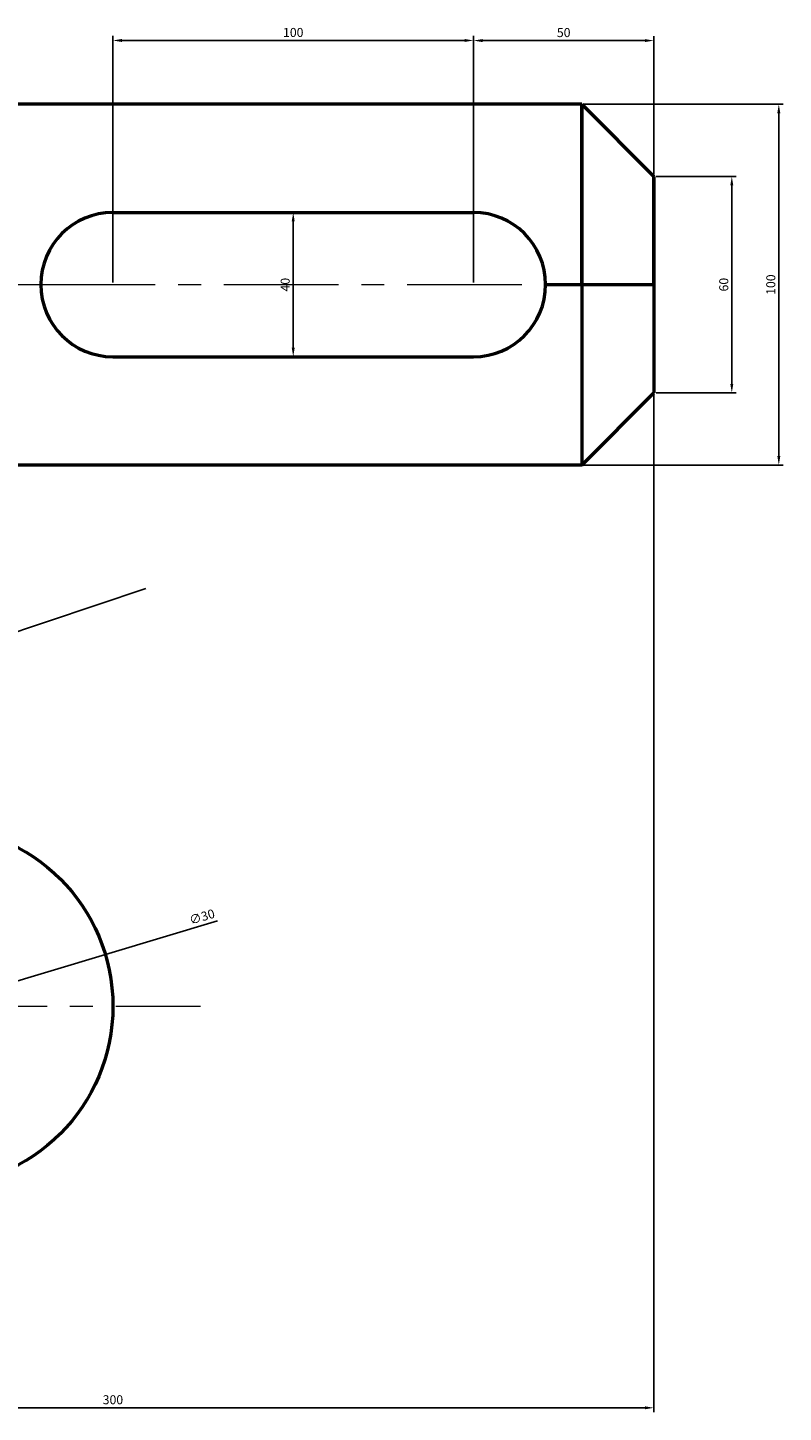
# Model space of a CAD drawing. Units: millimetres. Extents: x 107046 to 107591, y 80056 to 80641.
# Tile 2 of 3: x 107381 to 107591, y 80056 to 80440. Entities that reach past the tile are written whole.
import ezdxf

# ---------------------------------------------------------------- set-up
doc = ezdxf.new("R2010")
doc.units = ezdxf.units.MM
doc.linetypes.add('CENTER', pattern=[50.8, 31.75, -6.35, 6.35, -6.35])
for name, color, linetype, lineweight in [('M-CNTR', 1, 'CENTER', 18), ('M-DIMS', 2, 'Continuous', 25), ('M-OUTL', 7, 'Continuous', 50)]:
    doc.layers.add(name, color=color, linetype=linetype, lineweight=lineweight)
doc.styles.get("Standard").update_dxf_attribs({"font": 'arial.ttf'})
doc.dimstyles.new('ISO-25', dxfattribs={"dimtxt": 2.5, "dimasz": 2.5, "dimexe": 1.25, "dimexo": 0.625, "dimtad": 1, "dimtxsty": 'Standard', "dimcen": 2.5, "dimadec": 0, "dimazin": 0, "dimtfac": 1, "dimtmove": 0, "dimatfit": 3, "dimfxl": 1, "dimarcsym": 0})

# ---------------------------------------------------------------- blocks, each defined once
blk = doc.blocks.new('*D3')
at = {"layer": 'Defpoints', "color": 0, "transparency": 16777216}
for p in [(107255.14, 80368.78), (107555.14, 80368.78), (107555.14, 80057.52)]:
    blk.add_point(p, dxfattribs=at)
at = {"layer": 'M-DIMS', "color": 0, "lineweight": -2, "transparency": 16777216}
for p, q in [((107255.14, 80368.16), (107255.14, 80056.27)), ((107555.14, 80368.16), (107555.14, 80056.27)), ((107257.64, 80057.52), (107552.64, 80057.52))]:
    blk.add_line(p, q, dxfattribs=at)
at = {"layer": 'M-DIMS', "color": 0, "transparency": 16777216}
for points in [[(107257.64, 80057.94), (107257.64, 80057.11), (107255.14, 80057.52)], [(107552.64, 80057.94), (107552.64, 80057.11), (107555.14, 80057.52)]]:
    blk.add_solid(points, dxfattribs=at)
at = {"layer": 'M-DIMS', "color": 0, "transparency": 16777216, "insert": (107405.14, 80059.43), "char_height": 2.5, "attachment_point": 5}
blk.add_mtext('300', dxfattribs=at)
blk = doc.blocks.new('*D4')
at = {"layer": 'Defpoints', "color": 0, "transparency": 16777216}
for p in [(107505.14, 80436.44), (107405.14, 80368.78), (107505.14, 80368.78)]:
    blk.add_point(p, dxfattribs=at)
at = {"layer": 'M-DIMS', "color": 0, "lineweight": -2, "transparency": 16777216}
for p, q in [((107405.14, 80369.41), (107405.14, 80437.69)), ((107505.14, 80369.41), (107505.14, 80437.69)), ((107407.64, 80436.44), (107502.64, 80436.44))]:
    blk.add_line(p, q, dxfattribs=at)
at = {"layer": 'M-DIMS', "color": 0, "transparency": 16777216}
for points in [[(107407.64, 80436.86), (107407.64, 80436.03), (107405.14, 80436.44)], [(107502.64, 80436.86), (107502.64, 80436.03), (107505.14, 80436.44)]]:
    blk.add_solid(points, dxfattribs=at)
at = {"layer": 'M-DIMS', "color": 0, "transparency": 16777216, "insert": (107455.14, 80438.34), "char_height": 2.5, "attachment_point": 5}
blk.add_mtext('100', dxfattribs=at)
blk = doc.blocks.new('*D5')
at = {"layer": 'Defpoints', "color": 0, "transparency": 16777216}
for p in [(107455.14, 80388.78), (107455.14, 80348.78), (107455.14, 80348.78)]:
    blk.add_point(p, dxfattribs=at)
at = {"layer": 'M-DIMS', "color": 0, "lineweight": -2, "transparency": 16777216}
for p, q in [((107455.76, 80388.78), (107456.39, 80388.78)), ((107455.14, 80386.28), (107455.14, 80351.28)), ((107455.76, 80348.78), (107456.39, 80348.78))]:
    blk.add_line(p, q, dxfattribs=at)
at = {"layer": 'M-DIMS', "color": 0, "transparency": 16777216}
for points in [[(107454.72, 80386.28), (107455.55, 80386.28), (107455.14, 80388.78)], [(107454.72, 80351.28), (107455.55, 80351.28), (107455.14, 80348.78)]]:
    blk.add_solid(points, dxfattribs=at)
at = {"layer": 'M-DIMS', "color": 0, "transparency": 16777216, "insert": (107453.23, 80368.78), "char_height": 2.5, "attachment_point": 5, "rotation": 90}
blk.add_mtext('40', dxfattribs=at)
blk = doc.blocks.new('*D6')
at = {"layer": 'Defpoints', "color": 0, "transparency": 16777216}
for p in [(107505.14, 80436.44), (107555.14, 80436.41), (107555.14, 80398.78)]:
    blk.add_point(p, dxfattribs=at)
at = {"layer": 'M-DIMS', "color": 0, "lineweight": -2, "transparency": 16777216}
for p, q in [((107555.14, 80399.41), (107555.14, 80437.66)), ((107505.14, 80435.82), (107505.14, 80435.16)), ((107507.64, 80436.41), (107552.64, 80436.41))]:
    blk.add_line(p, q, dxfattribs=at)
at = {"layer": 'M-DIMS', "color": 0, "transparency": 16777216}
for points in [[(107507.64, 80436.83), (107507.64, 80436), (107505.14, 80436.41)], [(107552.64, 80436.83), (107552.64, 80436), (107555.14, 80436.41)]]:
    blk.add_solid(points, dxfattribs=at)
at = {"layer": 'M-DIMS', "color": 0, "transparency": 16777216, "insert": (107530.14, 80438.31), "char_height": 2.5, "attachment_point": 5}
blk.add_mtext('50', dxfattribs=at)
blk = doc.blocks.new('*D7')
at = {"layer": 'Defpoints', "color": 0, "transparency": 16777216}
for p in [(107555.14, 80398.78), (107555.14, 80338.78), (107576.76, 80338.78)]:
    blk.add_point(p, dxfattribs=at)
at = {"layer": 'M-DIMS', "color": 0, "lineweight": -2, "transparency": 16777216}
for p, q in [((107555.76, 80398.78), (107578.01, 80398.78)), ((107576.76, 80396.28), (107576.76, 80341.28)), ((107555.76, 80338.78), (107578.01, 80338.78))]:
    blk.add_line(p, q, dxfattribs=at)
at = {"layer": 'M-DIMS', "color": 0, "transparency": 16777216}
for points in [[(107576.34, 80396.28), (107577.17, 80396.28), (107576.76, 80398.78)], [(107576.34, 80341.28), (107577.17, 80341.28), (107576.76, 80338.78)]]:
    blk.add_solid(points, dxfattribs=at)
at = {"layer": 'M-DIMS', "color": 0, "transparency": 16777216, "insert": (107574.85, 80368.78), "char_height": 2.5, "attachment_point": 5, "rotation": 90}
blk.add_mtext('60', dxfattribs=at)
blk = doc.blocks.new('*D8')
at = {"layer": 'Defpoints', "color": 0, "transparency": 16777216}
for p in [(107535.14, 80418.78), (107535.14, 80318.78), (107589.79, 80318.78)]:
    blk.add_point(p, dxfattribs=at)
at = {"layer": 'M-DIMS', "color": 0, "lineweight": -2, "transparency": 16777216}
for p, q in [((107535.76, 80418.78), (107591.04, 80418.78)), ((107589.79, 80416.28), (107589.79, 80321.28)), ((107535.76, 80318.78), (107591.04, 80318.78))]:
    blk.add_line(p, q, dxfattribs=at)
at = {"layer": 'M-DIMS', "color": 0, "transparency": 16777216}
for points in [[(107589.38, 80416.28), (107590.21, 80416.28), (107589.79, 80418.78)], [(107589.38, 80321.28), (107590.21, 80321.28), (107589.79, 80318.78)]]:
    blk.add_solid(points, dxfattribs=at)
at = {"layer": 'M-DIMS', "color": 0, "transparency": 16777216, "insert": (107587.89, 80368.78), "char_height": 2.5, "attachment_point": 5, "rotation": 90}
blk.add_mtext('100', dxfattribs=at)
blk = doc.blocks.new('*D14')
at = {"layer": 'Defpoints', "color": 0, "transparency": 16777216}
for p in [(107414.23, 80284.58), (107338.38, 80259.13)]:
    blk.add_point(p, dxfattribs=at)
at = {"layer": 'M-DIMS', "color": 0, "lineweight": -2, "transparency": 16777216}
for p, q in [((107414.23, 80284.58), (107338.38, 80259.13)), ((107315.92, 80251.6), (107336.01, 80258.34))]:
    blk.add_line(p, q, dxfattribs=at)
at = {"layer": 'M-DIMS', "color": 0, "transparency": 16777216}
blk.add_solid([(107335.88, 80258.73), (107336.14, 80257.94), (107338.38, 80259.13)], dxfattribs=at)
at = {"layer": 'M-DIMS', "color": 0, "transparency": 16777216, "insert": (107318.73, 80254.55), "char_height": 2.5, "attachment_point": 5, "rotation": 18.5455}
blk.add_mtext('R80', dxfattribs=at)
blk = doc.blocks.new('*D16')
at = {"layer": 'Defpoints', "color": 0, "transparency": 16777216}
for p in [(107369.5, 80173.1), (107340.77, 80164.47)]:
    blk.add_point(p, dxfattribs=at)
at = {"layer": 'M-DIMS', "color": 0, "lineweight": -2, "transparency": 16777216}
for p, q in [((107434.11, 80192.49), (107371.9, 80173.81)), ((107340.77, 80164.47), (107369.5, 80173.1)), ((107338.38, 80163.75), (107335.98, 80163.03))]:
    blk.add_line(p, q, dxfattribs=at)
at = {"layer": 'M-DIMS', "color": 0, "transparency": 16777216}
for points in [[(107371.78, 80174.21), (107372.02, 80173.42), (107369.5, 80173.1)], [(107338.26, 80164.15), (107338.49, 80163.35), (107340.77, 80164.47)]]:
    blk.add_solid(points, dxfattribs=at)
at = {"layer": 'M-DIMS', "color": 0, "transparency": 16777216, "insert": (107429.93, 80193.29), "char_height": 2.5, "attachment_point": 5, "rotation": 16.7071}
blk.add_mtext('∅30', dxfattribs=at)

msp = doc.modelspace()

# ---------------------------------------------------------------- linework, layer by layer
at = {"layer": 'M-CNTR'}
for p, q in [((107255.136, 80368.784), (107385.136, 80368.784)), ((107385.136, 80368.784), (107525.136, 80368.784)), ((107555.136, 80368.784), (107525.136, 80368.784)), ((107555.136, 80368.784), (107535.136, 80368.784)), ((107355.136, 80168.784), (107429.433, 80168.784))]:
    msp.add_line(p, q, dxfattribs=at)
at = {"layer": 'M-OUTL'}
for p, q in [((107535.136, 80418.784), (107375.552, 80418.784)), ((107535.136, 80368.784), (107535.136, 80418.784)), ((107535.136, 80418.784), (107535.136, 80368.784)), ((107535.136, 80418.784), (107555.136, 80398.784)), ((107555.136, 80368.784), (107555.136, 80398.784)), ((107555.136, 80398.784), (107555.136, 80338.784)), ((107405.136, 80388.784), (107505.136, 80388.784)), ((107525.136, 80368.784), (107555.136, 80368.784)), ((107535.136, 80368.784), (107535.136, 80318.784)), ((107405.136, 80348.784), (107505.136, 80348.784)), ((107535.136, 80318.784), (107555.136, 80338.784)), ((107535.136, 80318.784), (107375.552, 80318.784))]:
    msp.add_line(p, q, dxfattribs=at)
msp.add_circle((107355.136, 80168.784), 50, dxfattribs=at)
for centre, start, end in [((107405.136, 80368.784), 90, 270), ((107505.136, 80368.784), 270, 90)]:
    msp.add_arc(centre, 20, start, end, dxfattribs=at)

# ---------------------------------------------------------------- dimensions: what is measured, and where the dimension line sits
at = {"layer": 'M-DIMS'}
for base, p1, p2, picture, middle in [((107505.136, 80436.443), (107405.136, 80368.784), (107505.136, 80368.784), '*D4', (107455.136, 80438.344)), ((107555.136, 80436.412), (107505.136, 80436.443), (107555.136, 80398.784), '*D6', (107530.136, 80438.313)), ((107555.136, 80057.524), (107255.136, 80368.784), (107555.136, 80368.784), '*D3', (107405.136, 80059.427))]:
    dim = msp.add_linear_dim(base=base, p1=p1, p2=p2, dimstyle='ISO-25', override={"dimclrd": 0, "dimclre": 0, "dimclrt": 0}, dxfattribs=at)
    dim.commit()
    dim.dimension.update_dxf_attribs({"geometry": picture, "text_midpoint": middle})
for base, p1, p2, picture, middle in [((107589.794, 80318.784), (107535.136, 80418.784), (107535.136, 80318.784), '*D8', (107587.892, 80368.784)), ((107576.756, 80338.784), (107555.136, 80398.784), (107555.136, 80338.784), '*D7', (107574.855, 80368.784)), ((107455.136, 80348.784), (107455.136, 80388.784), (107455.136, 80348.784), '*D5', (107453.235, 80368.784))]:
    dim = msp.add_linear_dim(base=base, p1=p1, p2=p2, angle=90, dimstyle='ISO-25', override={"dimclrd": 0, "dimclre": 0, "dimclrt": 0}, dxfattribs=at)
    dim.commit()
    dim.dimension.update_dxf_attribs({"geometry": picture, "text_midpoint": middle})
dim = msp.add_radius_dim(center=(107414.226, 80284.579), mpoint=(107338.38, 80259.134), dimstyle='ISO-25', override={"dimclrd": 0, "dimclre": 0, "dimclrt": 0}, dxfattribs=at)
dim.commit()
dim.dimension.update_dxf_attribs({"geometry": '*D14', "text_midpoint": (107319.339, 80252.746), "dimtype": 164})
dim = msp.add_diameter_dim_2p(p1=(107340.769, 80164.472), p2=(107369.503, 80173.096), dimstyle='ISO-25', override={"dimclrd": 0, "dimclre": 0, "dimclrt": 0}, dxfattribs=at)
dim.commit()
dim.dimension.update_dxf_attribs({"geometry": '*D16', "text_midpoint": (107430.499, 80191.404), "dimtype": 163})

doc.saveas('drawing.dxf')
